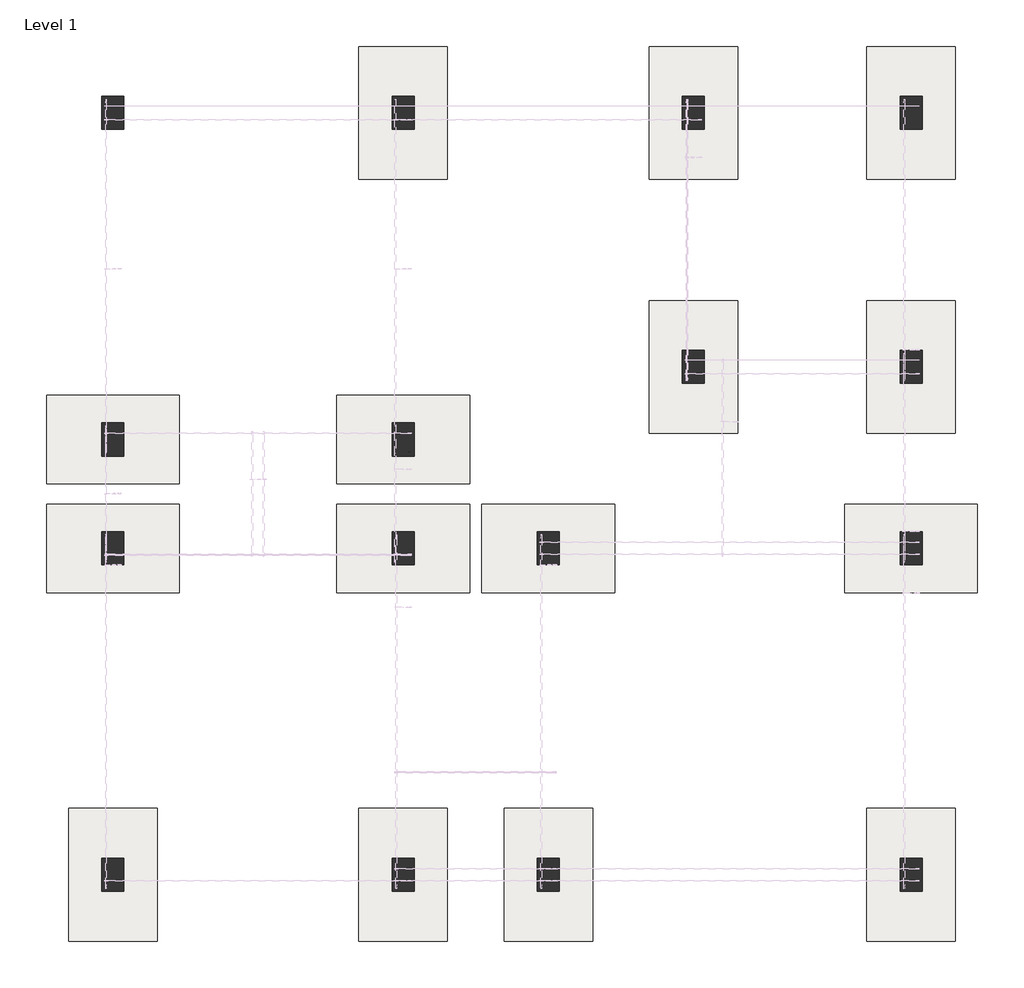
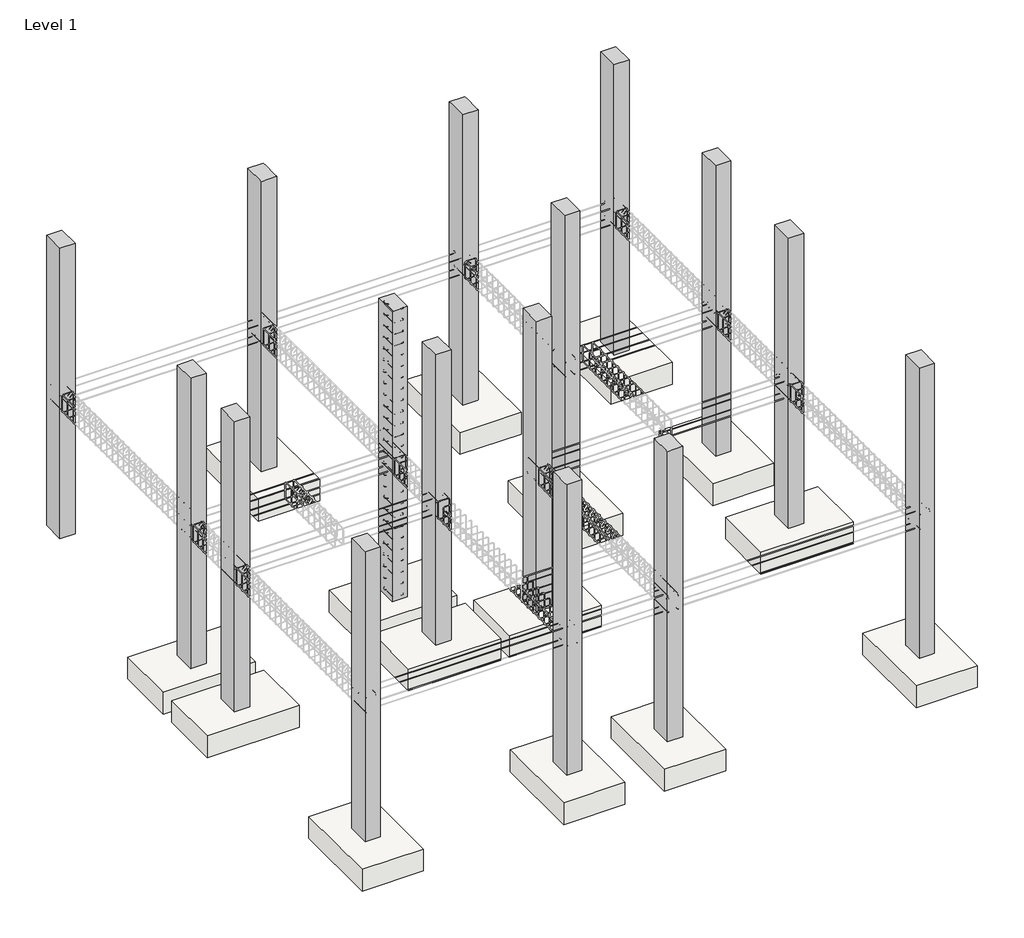
# One storey, part 1 of 5: 16 columns, 15 slabs.
"""IFC4 building model written with IfcOpenShell, lengths in millimetres."""

from ifc_helpers import new_model, si_unit, frame, origin, origin_with_axes, place, context, project, spatial, polyline, outline, extrude, faceted_brep, transform, mapped, element, save
from components import slab_5ba74754

model = new_model("IFC4")

# Units and contexts
model_context = context("Model", 3, world=origin())
ifc_project = project(units=[si_unit("LENGTHUNIT", "METRE", prefix="MILLI")], contexts=[model_context])

# Site, building, storey
site = spatial("IfcSite", under=ifc_project)
building = spatial("IfcBuilding", under=site)
storey = spatial("IfcBuildingStorey", under=building, Name="Level 1", Elevation=0.0)

# Columns
placement = place(None, origin())
element("IfcColumn", 1, ObjectType="Concrete-Rectangular-Column : 12 x 18", at=placement, inside=storey, context=model_context, shape_type="SweptSolid", body=[
    extrude(outline(polyline([(-15154.8215379, 8606.4267522), (-15154.8215379, 8149.2267522), (-15459.6215379, 8149.2267522), (-15459.6215379, 8606.4267522), (-15154.8215379, 8606.4267522)])), origin_with_axes(), (0.0, 0.0, 1.0), 6096.0),
])
element("IfcColumn", 2, ObjectType="Concrete-Rectangular-Column : 12 x 18", at=placement, inside=storey, context=model_context, shape_type="Brep", body=[
    faceted_brep([(-11154.8215379, 8606.4267522, 0.0), (-11154.8215379, 8149.2267522, 0.0), (-11459.6215379, 8149.2267522, 0.0), (-11459.6215379, 8606.4267522, 0.0), (-11154.8215379, 8606.4267522, 6096.0), (-11154.8215379, 8530.2267522, 6096.0), (-11154.8215379, 8225.4267522, 6096.0), (-11154.8215379, 8149.2267522, 6096.0), (-11459.6215379, 8149.2267522, 6096.0), (-11459.6215379, 8225.4267522, 6096.0), (-11459.6215379, 8530.2267522, 6096.0), (-11459.6215379, 8606.4267522, 6096.0)], [[[0, 1, 2, 3]], [[4, 5, 6, 7, 1, 0]], [[7, 8, 2, 1]], [[8, 9, 10, 11, 3, 2]], [[11, 4, 0, 3]], [[4, 11, 10, 9, 8, 7, 6, 5]]]),
])
element("IfcColumn", 3, ObjectType="Concrete-Rectangular-Column : 12 x 18", at=placement, inside=storey, context=model_context, shape_type="Brep", body=[
    faceted_brep([(-7154.8215379, 8606.4267522, 0.0), (-7154.8215379, 8149.2267522, 0.0), (-7459.6215379, 8149.2267522, 0.0), (-7459.6215379, 8606.4267522, 0.0), (-7154.8215379, 8606.4267522, 6096.0), (-7154.8215379, 8530.2267522, 6096.0), (-7154.8215379, 8225.4267522, 6096.0), (-7154.8215379, 8149.2267522, 6096.0), (-7459.6215379, 8149.2267522, 6096.0), (-7459.6215379, 8225.4267522, 6096.0), (-7459.6215379, 8530.2267522, 6096.0), (-7459.6215379, 8606.4267522, 6096.0)], [[[0, 1, 2, 3]], [[4, 5, 6, 7, 1, 0]], [[7, 8, 2, 1]], [[8, 9, 10, 11, 3, 2]], [[11, 4, 0, 3]], [[4, 11, 10, 9, 8, 7, 6, 5]]]),
])
element("IfcColumn", 4, ObjectType="Concrete-Rectangular-Column : 12 x 18", at=placement, inside=storey, context=model_context, shape_type="SweptSolid", body=[
    extrude(outline(polyline([(-4154.8215379, 8606.4267522), (-4154.8215379, 8149.2267522), (-4459.6215379, 8149.2267522), (-4459.6215379, 8606.4267522), (-4154.8215379, 8606.4267522)])), origin_with_axes(), (0.0, 0.0, 1.0), 6096.0),
])
element("IfcColumn", 5, ObjectType="Concrete-Rectangular-Column : 12 x 18", at=placement, inside=storey, context=model_context, shape_type="Brep", body=[
    faceted_brep([(-15154.8215379, 4106.4267522, 0.0), (-15154.8215379, 3649.2267522, 0.0), (-15459.6215379, 3649.2267522, 0.0), (-15459.6215379, 4106.4267522, 0.0), (-15154.8215379, 4106.4267522, 6096.0), (-15154.8215379, 3649.2267522, 6096.0), (-15154.8215379, 3649.2267522, 5638.8), (-15154.8215379, 3649.2267522, 3048.0), (-15154.8215379, 3649.2267522, 2590.8), (-15154.8215379, 4106.4267522, 2590.8), (-15154.8215379, 4106.4267522, 3048.0), (-15154.8215379, 4106.4267522, 5638.8), (-15459.6215379, 3649.2267522, 6096.0), (-15459.6215379, 3649.2267522, 5638.8), (-15459.6215379, 3649.2267522, 3048.0), (-15459.6215379, 3649.2267522, 2590.8), (-15459.6215379, 4106.4267522, 6096.0), (-15459.6215379, 4106.4267522, 5638.8), (-15459.6215379, 4106.4267522, 3048.0), (-15459.6215379, 4106.4267522, 2590.8)], [[[0, 1, 2, 3]], [[4, 5, 6, 7, 8, 1, 0, 9, 10, 11]], [[5, 12, 13, 14, 15, 2, 1, 8, 7, 6]], [[12, 16, 17, 18, 19, 3, 2, 15, 14, 13]], [[16, 4, 11, 10, 9, 0, 3, 19, 18, 17]], [[4, 16, 12, 5]]]),
])
element("IfcColumn", 6, ObjectType="Concrete-Rectangular-Column : 12 x 18", at=placement, inside=storey, context=model_context, shape_type="Brep", body=[
    faceted_brep([(-11154.8215379, 4106.4267522, 0.0), (-11154.8215379, 3649.2267522, 0.0), (-11459.6215379, 3649.2267522, 0.0), (-11459.6215379, 4106.4267522, 0.0), (-11154.8215379, 4106.4267522, 6096.0), (-11154.8215379, 3649.2267522, 6096.0), (-11154.8215379, 3649.2267522, 5638.8), (-11154.8215379, 3649.2267522, 3048.0), (-11154.8215379, 3649.2267522, 2590.8), (-11154.8215379, 4106.4267522, 2590.8), (-11154.8215379, 4106.4267522, 3048.0), (-11154.8215379, 4106.4267522, 5638.8), (-11459.6215379, 3649.2267522, 6096.0), (-11459.6215379, 3649.2267522, 5638.8), (-11459.6215379, 3649.2267522, 3048.0), (-11459.6215379, 3649.2267522, 2590.8), (-11459.6215379, 4106.4267522, 6096.0), (-11459.6215379, 4106.4267522, 5638.8), (-11459.6215379, 4106.4267522, 3048.0), (-11459.6215379, 4106.4267522, 2590.8)], [[[0, 1, 2, 3]], [[4, 5, 6, 7, 8, 1, 0, 9, 10, 11]], [[5, 12, 13, 14, 15, 2, 1, 8, 7, 6]], [[12, 16, 17, 18, 19, 3, 2, 15, 14, 13]], [[16, 4, 11, 10, 9, 0, 3, 19, 18, 17]], [[4, 16, 12, 5]]]),
])
element("IfcColumn", 7, ObjectType="Concrete-Rectangular-Column : 12 x 18", at=placement, inside=storey, context=model_context, shape_type="Brep", body=[
    faceted_brep([(-15154.8215379, 2606.4267522, 0.0), (-15154.8215379, 2149.2267522, 0.0), (-15459.6215379, 2149.2267522, 0.0), (-15459.6215379, 2606.4267522, 0.0), (-15154.8215379, 2606.4267522, 6096.0), (-15154.8215379, 2149.2267522, 6096.0), (-15154.8215379, 2149.2267522, 5638.8), (-15154.8215379, 2149.2267522, 3048.0), (-15154.8215379, 2149.2267522, 2590.8), (-15154.8215379, 2606.4267522, 2590.8), (-15154.8215379, 2606.4267522, 3048.0), (-15154.8215379, 2606.4267522, 5638.8), (-15459.6215379, 2149.2267522, 6096.0), (-15459.6215379, 2149.2267522, 5638.8), (-15459.6215379, 2149.2267522, 3048.0), (-15459.6215379, 2149.2267522, 2590.8), (-15459.6215379, 2606.4267522, 6096.0), (-15459.6215379, 2606.4267522, 5638.8), (-15459.6215379, 2606.4267522, 3048.0), (-15459.6215379, 2606.4267522, 2590.8)], [[[0, 1, 2, 3]], [[4, 5, 6, 7, 8, 1, 0, 9, 10, 11]], [[5, 12, 13, 14, 15, 2, 1, 8, 7, 6]], [[12, 16, 17, 18, 19, 3, 2, 15, 14, 13]], [[16, 4, 11, 10, 9, 0, 3, 19, 18, 17]], [[4, 16, 12, 5]]]),
])
element("IfcColumn", 8, ObjectType="Concrete-Rectangular-Column : 12 x 18", at=placement, inside=storey, context=model_context, shape_type="Brep", body=[
    faceted_brep([(-11154.8215379, 2606.4267522, 0.0), (-11154.8215379, 2149.2267522, 0.0), (-11459.6215379, 2149.2267522, 0.0), (-11459.6215379, 2606.4267522, 0.0), (-11154.8215379, 2606.4267522, 6096.0), (-11154.8215379, 2149.2267522, 6096.0), (-11154.8215379, 2149.2267522, 5638.8), (-11154.8215379, 2149.2267522, 3048.0), (-11154.8215379, 2149.2267522, 2590.8), (-11154.8215379, 2606.4267522, 2590.8), (-11154.8215379, 2606.4267522, 3048.0), (-11154.8215379, 2606.4267522, 5638.8), (-11459.6215379, 2149.2267522, 6096.0), (-11459.6215379, 2149.2267522, 5638.8), (-11459.6215379, 2149.2267522, 3048.0), (-11459.6215379, 2149.2267522, 2590.8), (-11459.6215379, 2606.4267522, 6096.0), (-11459.6215379, 2606.4267522, 5638.8), (-11459.6215379, 2606.4267522, 3048.0), (-11459.6215379, 2606.4267522, 2590.8)], [[[0, 1, 2, 3]], [[4, 5, 6, 7, 8, 1, 0, 9, 10, 11]], [[5, 12, 13, 14, 15, 2, 1, 8, 7, 6]], [[12, 16, 17, 18, 19, 3, 2, 15, 14, 13]], [[16, 4, 11, 10, 9, 0, 3, 19, 18, 17]], [[4, 16, 12, 5]]]),
])
element("IfcColumn", 9, ObjectType="Concrete-Rectangular-Column : 12 x 18", at=placement, inside=storey, context=model_context, shape_type="SweptSolid", body=[
    extrude(outline(polyline([(-15154.8215379, -1893.5732478), (-15154.8215379, -2350.7732478), (-15459.6215379, -2350.7732478), (-15459.6215379, -1893.5732478), (-15154.8215379, -1893.5732478)])), origin_with_axes(), (0.0, 0.0, 1.0), 6096.0),
])
element("IfcColumn", 10, ObjectType="Concrete-Rectangular-Column : 12 x 18", at=placement, inside=storey, context=model_context, shape_type="Brep", body=[
    faceted_brep([(-11154.8215379, -1893.5732478, 0.0), (-11154.8215379, -2350.7732478, 0.0), (-11459.6215379, -2350.7732478, 0.0), (-11459.6215379, -1893.5732478, 0.0), (-11154.8215379, -1893.5732478, 6096.0), (-11154.8215379, -1969.7732478, 6096.0), (-11154.8215379, -2274.5732478, 6096.0), (-11154.8215379, -2350.7732478, 6096.0), (-11459.6215379, -2350.7732478, 6096.0), (-11459.6215379, -2274.5732478, 6096.0), (-11459.6215379, -1969.7732478, 6096.0), (-11459.6215379, -1893.5732478, 6096.0)], [[[0, 1, 2, 3]], [[4, 5, 6, 7, 1, 0]], [[7, 8, 2, 1]], [[8, 9, 10, 11, 3, 2]], [[11, 4, 0, 3]], [[4, 11, 10, 9, 8, 7, 6, 5]]]),
])
element("IfcColumn", 11, ObjectType="Concrete-Rectangular-Column : 12 x 18", at=placement, inside=storey, context=model_context, shape_type="Brep", body=[
    faceted_brep([(-9154.8215379, -1893.5732478, 0.0), (-9154.8215379, -2350.7732478, 0.0), (-9459.6215379, -2350.7732478, 0.0), (-9459.6215379, -1893.5732478, 0.0), (-9154.8215379, -1893.5732478, 6096.0), (-9154.8215379, -1969.7732478, 6096.0), (-9154.8215379, -2274.5732478, 6096.0), (-9154.8215379, -2350.7732478, 6096.0), (-9459.6215379, -2350.7732478, 6096.0), (-9459.6215379, -2274.5732478, 6096.0), (-9459.6215379, -1969.7732478, 6096.0), (-9459.6215379, -1893.5732478, 6096.0)], [[[0, 1, 2, 3]], [[4, 5, 6, 7, 1, 0]], [[7, 8, 2, 1]], [[8, 9, 10, 11, 3, 2]], [[11, 4, 0, 3]], [[4, 11, 10, 9, 8, 7, 6, 5]]]),
])
element("IfcColumn", 12, ObjectType="Concrete-Rectangular-Column : 12 x 18", at=placement, inside=storey, context=model_context, shape_type="SweptSolid", body=[
    extrude(outline(polyline([(-4154.8215379, -1893.5732478), (-4154.8215379, -2350.7732478), (-4459.6215379, -2350.7732478), (-4459.6215379, -1893.5732478), (-4154.8215379, -1893.5732478)])), origin_with_axes(), (0.0, 0.0, 1.0), 6096.0),
])
element("IfcColumn", 13, ObjectType="Concrete-Rectangular-Column : 12 x 18", at=placement, inside=storey, context=model_context, shape_type="Brep", body=[
    faceted_brep([(-4154.8215379, 2606.4267522, 0.0), (-4154.8215379, 2149.2267522, 0.0), (-4459.6215379, 2149.2267522, 0.0), (-4459.6215379, 2606.4267522, 0.0), (-4154.8215379, 2606.4267522, 6096.0), (-4154.8215379, 2149.2267522, 6096.0), (-4154.8215379, 2149.2267522, 5638.8), (-4154.8215379, 2149.2267522, 3048.0), (-4154.8215379, 2149.2267522, 2590.8), (-4154.8215379, 2606.4267522, 2590.8), (-4154.8215379, 2606.4267522, 3048.0), (-4154.8215379, 2606.4267522, 5638.8), (-4459.6215379, 2149.2267522, 6096.0), (-4459.6215379, 2149.2267522, 5638.8), (-4459.6215379, 2149.2267522, 3048.0), (-4459.6215379, 2149.2267522, 2590.8), (-4459.6215379, 2606.4267522, 6096.0), (-4459.6215379, 2606.4267522, 5638.8), (-4459.6215379, 2606.4267522, 3048.0), (-4459.6215379, 2606.4267522, 2590.8)], [[[0, 1, 2, 3]], [[4, 5, 6, 7, 8, 1, 0, 9, 10, 11]], [[5, 12, 13, 14, 15, 2, 1, 8, 7, 6]], [[12, 16, 17, 18, 19, 3, 2, 15, 14, 13]], [[16, 4, 11, 10, 9, 0, 3, 19, 18, 17]], [[4, 16, 12, 5]]]),
])
element("IfcColumn", 14, ObjectType="Concrete-Rectangular-Column : 12 x 18", at=placement, inside=storey, context=model_context, shape_type="SweptSolid", body=[
    extrude(outline(polyline([(-9154.8215379, 2606.4267522), (-9154.8215379, 2149.2267522), (-9459.6215379, 2149.2267522), (-9459.6215379, 2606.4267522), (-9154.8215379, 2606.4267522)])), origin_with_axes(), (0.0, 0.0, 1.0), 6096.0),
])
element("IfcColumn", 15, ObjectType="Concrete-Rectangular-Column : 12 x 18", at=placement, inside=storey, context=model_context, shape_type="SweptSolid", body=[
    extrude(outline(polyline([(-7154.8215379, 5106.4267522), (-7154.8215379, 4649.2267522), (-7459.6215379, 4649.2267522), (-7459.6215379, 5106.4267522), (-7154.8215379, 5106.4267522)])), origin_with_axes(), (0.0, 0.0, 1.0), 6096.0),
])
element("IfcColumn", 16, ObjectType="Concrete-Rectangular-Column : 12 x 18", at=placement, inside=storey, context=model_context, shape_type="Brep", body=[
    faceted_brep([(-4154.8215379, 5106.4267522, 0.0), (-4154.8215379, 4649.2267522, 0.0), (-4459.6215379, 4649.2267522, 0.0), (-4459.6215379, 5106.4267522, 0.0), (-4154.8215379, 5106.4267522, 6096.0), (-4154.8215379, 4649.2267522, 6096.0), (-4154.8215379, 4649.2267522, 5638.8), (-4154.8215379, 4649.2267522, 3048.0), (-4154.8215379, 4649.2267522, 2590.8), (-4154.8215379, 5106.4267522, 2590.8), (-4154.8215379, 5106.4267522, 3048.0), (-4154.8215379, 5106.4267522, 5638.8), (-4459.6215379, 4649.2267522, 6096.0), (-4459.6215379, 4649.2267522, 5638.8), (-4459.6215379, 4649.2267522, 3048.0), (-4459.6215379, 4649.2267522, 2590.8), (-4459.6215379, 5106.4267522, 6096.0), (-4459.6215379, 5106.4267522, 5638.8), (-4459.6215379, 5106.4267522, 3048.0), (-4459.6215379, 5106.4267522, 2590.8)], [[[0, 1, 2, 3]], [[4, 5, 6, 7, 8, 1, 0, 9, 10, 11]], [[5, 12, 13, 14, 15, 2, 1, 8, 7, 6]], [[12, 16, 17, 18, 19, 3, 2, 15, 14, 13]], [[16, 4, 11, 10, 9, 0, 3, 19, 18, 17]], [[4, 16, 12, 5]]]),
])

# Slabs
element("IfcSlab", 17, ObjectType="Footing-Rectangular : 72\" x 48\" x 18\"", at=placement, inside=storey, context=model_context, shape_type="SweptSolid", body=[
    extrude(outline(polyline([(-16221.6215379, 2987.4267522), (-14392.8215379, 2987.4267522), (-14392.8215379, 1768.2267522), (-16221.6215379, 1768.2267522), (-16221.6215379, 2987.4267522)])), frame((0.0, 0.0, -457.2), z_axis=(0.0, 0.0, 1.0), x_axis=(1.0, 0.0, 0.0)), (0.0, 0.0, 1.0), 457.2),
])
slab_shape = slab_5ba74754(model_context)
element("IfcSlab", 18, ObjectType="Footing-Rectangular : 72\" x 48\" x 18\"", at=placement, inside=storey, context=model_context, shape_type="MappedRepresentation", body=[
    mapped(slab_shape, transform((-11307.2215379, 8377.8267522, 0.0), x_axis=(1.0, 0.0, 0.0), y_axis=(0.0, 1.0, 0.0), z_axis=(0.0, 0.0, 1.0))),
])
element("IfcSlab", 19, ObjectType="Footing-Rectangular : 72\" x 48\" x 18\"", at=placement, inside=storey, context=model_context, shape_type="MappedRepresentation", body=[
    mapped(slab_shape, transform((-7307.2215379, 8377.8267522, 0.0), x_axis=(1.0, 0.0, 0.0), y_axis=(0.0, 1.0, 0.0), z_axis=(0.0, 0.0, 1.0))),
])
element("IfcSlab", 20, ObjectType="Footing-Rectangular : 72\" x 48\" x 18\"", at=placement, inside=storey, context=model_context, shape_type="MappedRepresentation", body=[
    mapped(slab_shape, transform((-4307.2215379, 8377.8267522, 0.0), x_axis=(1.0, 0.0, 0.0), y_axis=(0.0, 1.0, 0.0), z_axis=(0.0, 0.0, 1.0))),
])
element("IfcSlab", 21, ObjectType="Footing-Rectangular : 72\" x 48\" x 18\"", at=placement, inside=storey, context=model_context, shape_type="MappedRepresentation", body=[
    mapped(slab_shape, transform((-4307.2215379, 4877.8267522, 0.0), x_axis=(1.0, 0.0, 0.0), y_axis=(0.0, 1.0, 0.0), z_axis=(0.0, 0.0, 1.0))),
])
element("IfcSlab", 22, ObjectType="Footing-Rectangular : 72\" x 48\" x 18\"", at=placement, inside=storey, context=model_context, shape_type="MappedRepresentation", body=[
    mapped(slab_shape, transform((-7307.2215379, 4877.8267522, 0.0), x_axis=(1.0, 0.0, 0.0), y_axis=(0.0, 1.0, 0.0), z_axis=(0.0, 0.0, 1.0))),
])
element("IfcSlab", 23, ObjectType="Footing-Rectangular : 72\" x 48\" x 18\"", at=placement, inside=storey, context=model_context, shape_type="MappedRepresentation", body=[
    mapped(slab_shape, transform((-15307.2215379, 3877.8267522, 0.0), x_axis=(0.0, 1.0, 0.0), y_axis=(-1.0, 0.0, 0.0), z_axis=(0.0, 0.0, 1.0))),
])
element("IfcSlab", 24, ObjectType="Footing-Rectangular : 72\" x 48\" x 18\"", at=placement, inside=storey, context=model_context, shape_type="MappedRepresentation", body=[
    mapped(slab_shape, transform((-11307.2215379, 3877.8267522, 0.0), x_axis=(0.0, 1.0, 0.0), y_axis=(-1.0, 0.0, 0.0), z_axis=(0.0, 0.0, 1.0))),
])
element("IfcSlab", 25, ObjectType="Footing-Rectangular : 72\" x 48\" x 18\"", at=placement, inside=storey, context=model_context, shape_type="MappedRepresentation", body=[
    mapped(slab_shape, transform((-11307.2215379, 2377.8267522, 0.0), x_axis=(0.0, 1.0, 0.0), y_axis=(-1.0, 0.0, 0.0), z_axis=(0.0, 0.0, 1.0))),
])
element("IfcSlab", 26, ObjectType="Footing-Rectangular : 72\" x 48\" x 18\"", at=placement, inside=storey, context=model_context, shape_type="MappedRepresentation", body=[
    mapped(slab_shape, transform((-9307.2215379, 2377.8267522, 0.0), x_axis=(0.0, 1.0, 0.0), y_axis=(-1.0, 0.0, 0.0), z_axis=(0.0, 0.0, 1.0))),
])
element("IfcSlab", 27, ObjectType="Footing-Rectangular : 72\" x 48\" x 18\"", at=placement, inside=storey, context=model_context, shape_type="MappedRepresentation", body=[
    mapped(slab_shape, transform((-4307.2215379, 2377.8267522, 0.0), x_axis=(0.0, 1.0, 0.0), y_axis=(-1.0, 0.0, 0.0), z_axis=(0.0, 0.0, 1.0))),
])
element("IfcSlab", 28, ObjectType="Footing-Rectangular : 72\" x 48\" x 18\"", at=placement, inside=storey, context=model_context, shape_type="MappedRepresentation", body=[
    mapped(slab_shape, transform((-4307.2215379, -2122.1732478, 0.0), x_axis=(-1.0, 0.0, 0.0), y_axis=(0.0, -1.0, 0.0), z_axis=(0.0, 0.0, 1.0))),
])
element("IfcSlab", 29, ObjectType="Footing-Rectangular : 72\" x 48\" x 18\"", at=placement, inside=storey, context=model_context, shape_type="MappedRepresentation", body=[
    mapped(slab_shape, transform((-9307.2215379, -2122.1732478, 0.0), x_axis=(-1.0, 0.0, 0.0), y_axis=(0.0, -1.0, 0.0), z_axis=(0.0, 0.0, 1.0))),
])
element("IfcSlab", 30, ObjectType="Footing-Rectangular : 72\" x 48\" x 18\"", at=placement, inside=storey, context=model_context, shape_type="MappedRepresentation", body=[
    mapped(slab_shape, transform((-11307.2215379, -2122.1732478, 0.0), x_axis=(-1.0, 0.0, 0.0), y_axis=(0.0, -1.0, 0.0), z_axis=(0.0, 0.0, 1.0))),
])
element("IfcSlab", 31, ObjectType="Footing-Rectangular : 72\" x 48\" x 18\"", at=placement, inside=storey, context=model_context, shape_type="MappedRepresentation", body=[
    mapped(slab_shape, transform((-15307.2215379, -2122.1732478, 0.0), x_axis=(-1.0, 0.0, 0.0), y_axis=(0.0, -1.0, 0.0), z_axis=(0.0, 0.0, 1.0))),
])

save(model, "model.ifc")

# Revit data of these elements
# Type "Concrete-Rectangular-Column : 12 x 18"
#   Assembly Code = "B10"
#   b = 1' - 0"
#   h = 1' - 6"
#   Structural Material [instance default] = Concrete, Cast-in-Place gray
# Type "Footing-Rectangular : 72\" x 48\" x 18\""
#   Assembly Code = "A1010100"
#   Width = 4' - 0"
#   Length = 6' - 0"
#   Foundation Thickness = 1' - 6"
#   Structural Material [instance default] = Concrete, Cast-in-Place gray
# Elements 1, 2, 3, 4, 5, 6, 7, 8, 9, 10, 11, 12, 13, 14, 15, 16 (IfcColumn, "Concrete-Rectangular-Column : 12 x 18")
#   Structural Material = Concrete, Cast-in-Place gray
#   Phase Created = New Construction
#   Materials on its faces: "Concrete, Cast-in-Place gray"
# Elements 17, 18, 19, 20, 21, 22, 23, 24, 25, 26, 27, 28, 29, 30, 31 (IfcSlab, "Footing-Rectangular : 72\" x 48\" x 18\"")
#   Structural Material = Concrete, Cast-in-Place gray
#   Phase Created = New Construction
#   Materials on its faces: "Concrete, Cast-in-Place gray"
# Materials
#   "Concrete, Cast-in-Place gray": class "Concrete", colour RGB 192 192 192, transparency 0, Description = "Cast-in-place concrete", Cost = 0
